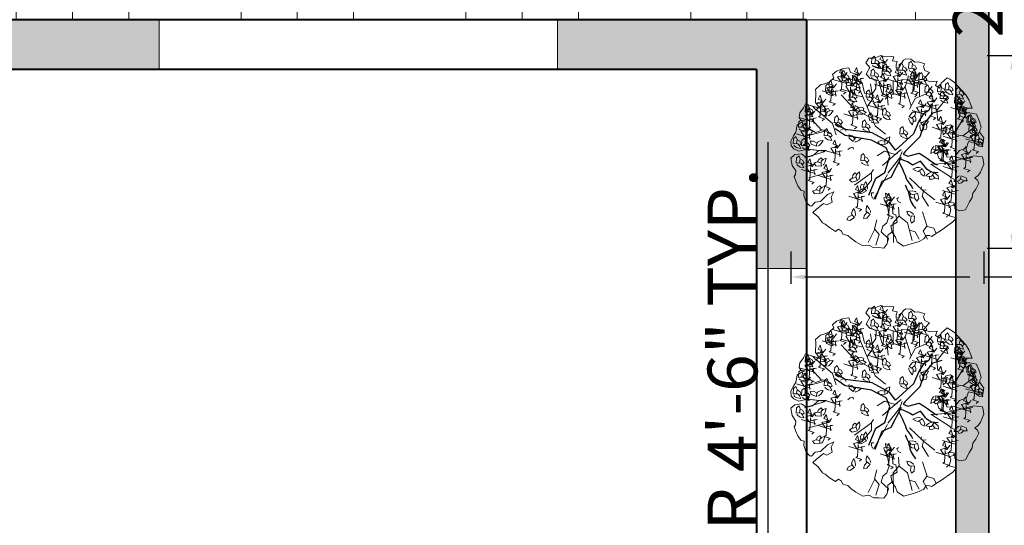
# Model space of a CAD drawing. Units: inches. Extents: x 2337 to 3570, y 1258 to 1938.
# Tile 27 of 30: x 3293 to 3471, y 1673 to 1764. Entities that reach past the tile are written whole.
import ezdxf

# ---------------------------------------------------------------- set-up
doc = ezdxf.new("R2010")
doc.units = ezdxf.units.IN
for name, color, linetype, lineweight in [('A-ANNO-DIMS', 2, 'Continuous', 18), ('A-FLOR-EDGE', 8, 'Continuous', 20), ('A-FLOR-PATT', 252, 'Continuous', 13), ('A-GLAZ', 4, 'Continuous', 18), ('A-WALL', 7, 'Continuous', 40), ('ARBOL', 74, 'Continuous', 13), ('C-PROP', 7, 'Continuous', 35)]:
    doc.layers.add(name, color=color, linetype=linetype, lineweight=lineweight)
doc.layers.add('A-WALL-PATT', color=18, linetype='Continuous', lineweight=13, true_color=0x000000)
doc.layers.add('C-PROP-PATT', color=251, linetype='Continuous', lineweight=13, true_color=0x636466)
doc.layers.add('TALLO', color=36, linetype='Continuous')
doc.styles.get("Standard").update_dxf_attribs({"font": 'arial.ttf'})
doc.dimstyles.new('ISO-25', dxfattribs={"dimtxt": 9, "dimasz": 2.5, "dimexe": 1.25, "dimexo": 0.625, "dimtad": 1, "dimdec": 1, "dimlunit": 3, "dimtxsty": 'Standard', "dimcen": 2.5, "dimadec": 0, "dimazin": 0, "dimtfac": 1, "dimtdec": 1, "dimtmove": 0, "dimatfit": 3, "dimfxl": 1, "dimarcsym": 0})

# ---------------------------------------------------------------- blocks, each defined once
blk = doc.blocks.new('fresno')
at = {"layer": 'ARBOL'}
for p, q in [((2.96, 0.991), (3.575, 1.984)), ((-3.638, 1.194), (-4.164, 1.76)), ((-1.151, -0.932), (-1.99, -1.556)), ((-0.974, -3.757), (-1.31, -4.423))]:
    blk.add_line(p, q, dxfattribs=at)
blk.add_lwpolyline([(0.823, 4.745), (0.566, 4.764), (0.459, 4.687), (0.336, 4.518), (0.233, 4.322), (0.087, 4.298), (0.091, 4.464), (0.14, 4.621), (-0.09, 4.659), (-0.033, 4.863), (-0.264, 4.901), (-0.483, 4.866), (-0.686, 4.924), (-1.021, 4.801), (-1.288, 4.8), (-1.431, 4.563), (-1.234, 4.327), (-1.406, 4), (-1.205, 3.778), (-0.909, 3.705), (-0.931, 3.283), (-1.122, 2.983), (-1.491, 3.043), (-1.619, 3.562), (-1.9, 3.727), (-1.851, 3.982), (-2.197, 4.084), (-2.278, 4.31), (-2.543, 4.283), (-2.896, 4.152), (-3.091, 3.971), (-3.022, 3.817), (-3.244, 3.617), (-3.424, 3.528), (-3.697, 3.455), (-3.946, 3.236), (-3.922, 3.09), (-3.94, 2.548), (-3.617, 2.495), (-3.927, 2.19), (-4.062, 2.379), (-4.443, 2.512), (-4.546, 2.316), (-4.73, 2.062), (-4.767, 1.832), (-4.671, 1.698), (-4.486, 1.667), (-4.693, 1.559), (-4.854, 1.444), (-4.934, 1.102), (-5.037, 0.905), (-5.175, 0.644), (-5.166, 0.406), (-5.024, 0.264), (-4.781, 0.153), (-4.363, 0.249), (-4.014, 0.215), (-3.783, 0.177), (-3.46, 0.124), (-3.733, 0.051), (-4.132, -0.073), (-4.404, -0.146), (-4.639, 0.011), (-4.977, -0.028), (-5.172, -0.209), (-5.113, -0.574), (-4.921, -0.843), (-4.951, -1.027), (-5.012, -1.112), (-4.95, -1.311), (-4.83, -1.592), (-4.676, -1.807), (-4.518, -1.856), (-4.529, -2.068), (-4.417, -2.394), (-4.236, -2.59), (-4.143, -2.605), (-3.967, -2.397), (-3.703, -2.37), (-3.339, -2.027), (-3.032, -1.889), (-3.169, -2.15), (-3.115, -2.396), (-3.376, -2.542), (-3.552, -2.466), (-3.909, -2.762), (-4.077, -2.924), (-3.804, -3.135), (-3.592, -3.43), (-3.461, -3.499), (-3.253, -3.676), (-2.953, -3.867), (-2.792, -3.752), (-2.642, -3.848), (-2.572, -4.001), (-2.323, -4.066), (-2.18, -4.208), (-1.926, -4.392), (-1.58, -4.591), (-1.288, -4.545), (-1.027, -4.683), (-0.788, -4.675), (-0.531, -4.693), (-0.382, -4.505), (-0.29, -4.236), (-0.66, -3.891), (-0.588, -3.595), (-0.374, -3.441), (-0.267, -3.079), (-0.368, -2.541), (-0.208, -2.426), (-0.099, -2.633), (-0.087, -2.991), (0.071, -3.04), (0.129, -3.405), (-0.185, -3.59), (-0.119, -3.909), (0.055, -4.151), (0.136, -4.377), (0.456, -4.596), (0.828, -4.491), (1.227, -4.368), (1.461, -4.241), (1.583, -4.071), (1.748, -4.075), (1.86, -4.117), (2.101, -3.944), (2.308, -3.836), (2.925, -3.393), (3.101, -3.185), (2.74, -3.078), (2.812, -2.782), (2.769, -2.61), (3.015, -2.555), (3.012, -2.721), (3.254, -2.832), (3.546, -2.785), (3.752, -2.393), (3.882, -2.177), (3.92, -1.947), (4.069, -1.758), (4.214, -1.451), (4.144, -1.297), (4.021, -1.182), (4.182, -1.067), (4.304, -0.897), (4.464, -0.497), (4.429, -0.279), (4.406, -0.133), (3.964, -0.083), (3.074, -0.315), (2.582, -0.424), (2.217, -0.197), (2.136, 0.029), (2.462, 0.141), (2.628, -0.147), (3.012, -0.116), (3.249, 0.177), (3.602, 0.308), (3.701, 0.623), (4.089, 0.535), (4.404, 0.436), (4.464, 0.805), (4.272, 1.074), (4.267, 1.193), (4.336, 1.324), (4.243, 1.623), (4.092, 2.003), (3.769, 2.057), (3.485, 2.056), (3.642, 2.291), (3.88, 2.299), (3.71, 2.706), (3.563, 2.967), (3.201, 3.358), (3.001, 3.581), (2.766, 3.738), (2.635, 3.807), (2.332, 3.549), (2.268, 3.299), (2.052, 3.429), (2.136, 3.652), (1.798, 3.613), (1.437, 3.72), (1.755, 4.071), (1.513, 4.182), (1.451, 4.381), (1.519, 4.512), (1.204, 4.611), (1.012, 4.596)], close=True, dxfattribs=at)
for points in [[(-0.346, 4.735), (-0.501, 4.528), (-0.605, 4.545), (-0.605, 4.614), (-0.519, 4.563), (-0.622, 4.925), (-0.726, 4.735), (-0.484, 4.632), (-0.622, 4.58), (-0.829, 4.528), (-0.657, 4.27), (-1.053, 4.39), (-0.363, 4.183), (-0.381, 4.114), (-0.415, 4.373), (-0.26, 4.39), (-0.57, 4.321), (-0.588, 4.476), (-0.622, 3.89), (-0.708, 3.839), (-0.398, 3.735), (-0.467, 3.701), (-0.519, 3.649)], [(-1.104, 4.45), (-1.063, 4.399), (-0.939, 4.325), (-0.757, 4.285), (-0.82, 4.431), (-0.903, 4.527), (-1.075, 4.533), (-1.143, 4.521), (-1.126, 4.792), (-1.002, 4.891), (-0.939, 4.738), (-0.975, 4.535)], [(-0.935, 4.717), (-0.809, 4.65), (-0.736, 4.529), (-0.824, 4.459)], [(-0.521, 4.069), (-0.48, 4.018), (-0.356, 3.944), (-0.174, 3.904), (-0.237, 4.051), (-0.32, 4.146), (-0.492, 4.152), (-0.56, 4.14), (-0.543, 4.411), (-0.419, 4.511), (-0.356, 4.357), (-0.392, 4.154)], [(0.263, 4.114), (0.304, 4.063), (0.429, 3.989), (0.611, 3.948), (0.547, 4.095), (0.465, 4.191), (0.293, 4.197), (0.225, 4.185), (0.242, 4.456), (0.366, 4.555), (0.428, 4.402), (0.393, 4.199)], [(0.734, 4.203), (0.775, 4.152), (0.9, 4.078), (1.082, 4.038), (1.018, 4.185), (0.936, 4.281), (0.763, 4.287), (0.696, 4.274), (0.712, 4.546), (0.837, 4.645), (0.899, 4.491), (0.863, 4.289)], [(0.904, 4.471), (1.029, 4.404), (1.102, 4.282), (1.015, 4.212)], [(-2.368, 4.073), (-2.523, 3.866), (-2.627, 3.883), (-2.627, 3.952), (-2.541, 3.9), (-2.644, 4.262), (-2.748, 4.073), (-2.506, 3.969), (-2.644, 3.918), (-2.851, 3.866), (-2.679, 3.607), (-3.075, 3.728), (-2.385, 3.521), (-2.403, 3.452), (-2.437, 3.711), (-2.282, 3.728), (-2.592, 3.659), (-2.61, 3.814), (-2.644, 3.228), (-2.73, 3.176), (-2.42, 3.073), (-2.489, 3.038), (-2.541, 2.987)], [(-2.629, 3.733), (-2.588, 3.682), (-2.463, 3.608), (-2.281, 3.568), (-2.345, 3.715), (-2.427, 3.81), (-2.6, 3.816), (-2.667, 3.804), (-2.651, 4.075), (-2.526, 4.175), (-2.464, 4.021), (-2.5, 3.818)], [(-2.459, 4), (-2.334, 3.933), (-2.261, 3.812), (-2.348, 3.742)], [(-1.623, 4.132), (-1.778, 3.925), (-1.882, 3.942), (-1.882, 4.011), (-1.795, 3.959), (-1.899, 4.321), (-2.002, 4.132), (-1.761, 4.028), (-1.899, 3.977), (-2.106, 3.925), (-1.933, 3.666), (-2.33, 3.787), (-1.64, 3.58), (-1.657, 3.511), (-1.692, 3.77), (-1.537, 3.787), (-1.847, 3.718), (-1.864, 3.873), (-1.899, 3.287), (-1.985, 3.235), (-1.675, 3.132), (-1.744, 3.097), (-1.795, 3.046)], [(-1.149, 3.822), (-1.108, 3.771), (-0.983, 3.697), (-0.802, 3.657), (-0.865, 3.804), (-0.948, 3.9), (-1.12, 3.906), (-1.188, 3.893), (-1.171, 4.165), (-1.047, 4.264), (-0.984, 4.111), (-1.02, 3.908)], [(-0.287, 3.833), (-0.442, 3.626), (-0.546, 3.643), (-0.546, 3.712), (-0.46, 3.661), (-0.563, 4.023), (-0.667, 3.833), (-0.425, 3.73), (-0.563, 3.678), (-0.77, 3.626), (-0.598, 3.367), (-0.995, 3.488), (-0.304, 3.281), (-0.322, 3.212), (-0.356, 3.471), (-0.201, 3.488), (-0.511, 3.419), (-0.529, 3.574), (-0.563, 2.988), (-0.649, 2.936), (-0.339, 2.833), (-0.408, 2.799), (-0.46, 2.747)], [(-0.98, 4.09), (-0.854, 4.023), (-0.781, 3.901), (-0.869, 3.831)], [(-0.352, 4.337), (-0.226, 4.269), (-0.153, 4.148), (-0.241, 4.078)], [(0.413, 4.08), (0.258, 3.873), (0.154, 3.89), (0.154, 3.959), (0.241, 3.908), (0.137, 4.27), (0.034, 4.08), (0.275, 3.977), (0.137, 3.925), (-0.07, 3.873), (0.103, 3.614), (-0.294, 3.735), (0.396, 3.528), (0.379, 3.459), (0.344, 3.718), (0.499, 3.735), (0.189, 3.666), (0.172, 3.821), (0.137, 3.235), (0.051, 3.183), (0.361, 3.08), (0.292, 3.046), (0.241, 2.994)], [(0.433, 4.381), (0.558, 4.314), (0.631, 4.193), (0.544, 4.122)], [(1.189, 3.942), (1.034, 3.735), (0.931, 3.752), (0.931, 3.821), (1.017, 3.77), (0.913, 4.132), (0.81, 3.942), (1.051, 3.839), (0.913, 3.787), (0.706, 3.735), (0.879, 3.477), (0.482, 3.597), (1.172, 3.39), (1.155, 3.321), (1.12, 3.58), (1.276, 3.597), (0.965, 3.528), (0.948, 3.683), (0.913, 3.097), (0.827, 3.046), (1.138, 2.942), (1.069, 2.908), (1.017, 2.856)], [(1.259, 4.08), (1.103, 3.873), (1, 3.89), (1, 3.959), (1.086, 3.908), (0.982, 4.27), (0.879, 4.08), (1.12, 3.977), (0.982, 3.925), (0.775, 3.873), (0.948, 3.614), (0.551, 3.735), (1.241, 3.528), (1.224, 3.459), (1.189, 3.718), (1.345, 3.735), (1.034, 3.666), (1.017, 3.821), (0.982, 3.235), (0.896, 3.183), (1.207, 3.08), (1.138, 3.046), (1.086, 2.994)], [(1.25, 3.643), (1.291, 3.592), (1.416, 3.518), (1.597, 3.478), (1.534, 3.625), (1.451, 3.721), (1.279, 3.727), (1.211, 3.714), (1.228, 3.985), (1.352, 4.085), (1.415, 3.931), (1.379, 3.729)], [(-2.898, 3.511), (-3.053, 3.304), (-3.157, 3.321), (-3.157, 3.39), (-3.071, 3.339), (-3.174, 3.701), (-3.278, 3.511), (-3.036, 3.408), (-3.174, 3.356), (-3.381, 3.304), (-3.209, 3.046), (-3.605, 3.166), (-2.915, 2.959), (-2.932, 2.89), (-2.967, 3.149), (-2.812, 3.166), (-3.122, 3.097), (-3.14, 3.253), (-3.174, 2.666), (-3.26, 2.615), (-2.95, 2.511), (-3.019, 2.477), (-3.071, 2.425)], [(-3.413, 3.083), (-3.373, 3.032), (-3.248, 2.958), (-3.066, 2.918), (-3.129, 3.065), (-3.212, 3.161), (-3.384, 3.167), (-3.452, 3.154), (-3.435, 3.425), (-3.311, 3.525), (-3.248, 3.371), (-3.284, 3.169)], [(-1.951, 3.597), (-2.106, 3.39), (-2.209, 3.408), (-2.209, 3.477), (-2.123, 3.425), (-2.227, 3.787), (-2.33, 3.597), (-2.089, 3.494), (-2.227, 3.442), (-2.434, 3.39), (-2.261, 3.132), (-2.658, 3.252), (-1.968, 3.046), (-1.985, 2.977), (-2.02, 3.235), (-1.864, 3.252), (-2.175, 3.183), (-2.192, 3.339), (-2.227, 2.752), (-2.313, 2.701), (-2.002, 2.597), (-2.071, 2.563), (-2.123, 2.511)], [(-2.068, 3.464), (-2.027, 3.413), (-1.903, 3.339), (-1.721, 3.299), (-1.784, 3.446), (-1.867, 3.542), (-2.039, 3.547), (-2.107, 3.535), (-2.09, 3.806), (-1.966, 3.906), (-1.903, 3.752), (-1.939, 3.55)], [(-1.899, 3.732), (-1.773, 3.664), (-1.7, 3.543), (-1.788, 3.473)], [(-1.367, 2.367), (-1.081, 2.78), (-1.193, 3.514)], [(-0.923, 3.449), (-0.951, 3.425), (-0.93, 3.313)], [(-0.358, 2.895), (-0.615, 3.037), (-0.783, 3.596)], [(-0.063, 3.671), (-0.069, 3.151), (-0.364, 2.965), (-0.319, 2.449)], [(0.558, 3.402), (0.403, 3.195), (0.299, 3.212), (0.299, 3.281), (0.386, 3.23), (0.282, 3.592), (0.179, 3.402), (0.42, 3.299), (0.282, 3.247), (0.075, 3.195), (0.248, 2.936), (-0.149, 3.057), (0.541, 2.85), (0.524, 2.781), (0.489, 3.04), (0.644, 3.057), (0.334, 2.988), (0.317, 3.143), (0.282, 2.557), (0.196, 2.505), (0.506, 2.402), (0.437, 2.368), (0.386, 2.316)], [(0.837, 2.414), (0.533, 3.352), (0.697, 3.906)], [(1.259, 2.882), (1.254, 3.446), (1.381, 3.636)], [(1.419, 3.911), (1.545, 3.844), (1.618, 3.722), (1.53, 3.652)], [(1.564, 3.016), (1.605, 2.965), (1.729, 2.891), (1.911, 2.851), (1.848, 2.998), (1.765, 3.094), (1.593, 3.099), (1.525, 3.087), (1.542, 3.358), (1.666, 3.458), (1.729, 3.304), (1.693, 3.102)], [(2.191, 3.038), (2.232, 2.987), (2.357, 2.913), (2.539, 2.873), (2.475, 3.02), (2.393, 3.116), (2.221, 3.122), (2.153, 3.109), (2.17, 3.381), (2.294, 3.48), (2.356, 3.326), (2.321, 3.124)], [(2.573, 3.128), (2.613, 3.077), (2.738, 3.003), (2.92, 2.963), (2.857, 3.11), (2.774, 3.205), (2.602, 3.211), (2.534, 3.199), (2.551, 3.47), (2.675, 3.57), (2.738, 3.416), (2.702, 3.214)], [(-3.244, 3.351), (-3.118, 3.284), (-3.045, 3.162), (-3.133, 3.092)], [(-1.112, 1.773), (-2.014, 2.265), (-2.654, 2.957)], [(-2.225, 2.77), (-2.184, 2.718), (-2.06, 2.645), (-1.878, 2.604), (-1.941, 2.751), (-2.024, 2.847), (-2.196, 2.853), (-2.264, 2.84), (-2.247, 3.112), (-2.123, 3.211), (-2.06, 3.058), (-2.096, 2.855)], [(-1.575, 2.854), (-2.052, 2.969), (-2.2, 3.178)], [(-2.056, 3.037), (-1.93, 2.97), (-1.857, 2.849), (-1.945, 2.778)], [(-0.448, 1), (-0.961, 1.419), (-1.784, 3.341)], [(-1.373, 2.77), (-1.332, 2.718), (-1.208, 2.645), (-1.026, 2.604), (-1.089, 2.751), (-1.172, 2.847), (-1.344, 2.853), (-1.412, 2.84), (-1.395, 3.112), (-1.271, 3.211), (-1.208, 3.058), (-1.244, 2.855)], [(-0.57, 2.77), (-0.726, 2.563), (-0.829, 2.58), (-0.829, 2.649), (-0.743, 2.597), (-0.846, 2.959), (-0.95, 2.77), (-0.708, 2.666), (-0.846, 2.615), (-1.053, 2.563), (-0.881, 2.304), (-1.278, 2.425), (-0.588, 2.218), (-0.605, 2.149), (-0.639, 2.408), (-0.484, 2.425), (-0.795, 2.356), (-0.812, 2.511), (-0.846, 1.925), (-0.933, 1.873), (-0.622, 1.77), (-0.691, 1.735), (-0.743, 1.684)], [(-1.204, 3.037), (-1.078, 2.97), (-1.005, 2.849), (-1.093, 2.778)], [(-0.41, 3.035), (-0.387, 2.974), (-0.291, 2.865), (-0.131, 2.771), (-0.146, 2.93), (-0.195, 3.047), (-0.357, 3.106), (-0.425, 3.115), (-0.325, 3.368), (-0.176, 3.424), (-0.164, 3.258), (-0.261, 3.077)], [(-0.166, 3.238), (-0.068, 3.135), (-0.036, 2.997), (-0.141, 2.957)], [(0.746, 2.242), (1.034, 2.786), (1.584, 3.019), (1.879, 3.374)], [(2.121, 2.804), (1.966, 2.597), (1.862, 2.615), (1.862, 2.683), (1.949, 2.632), (1.845, 2.994), (1.742, 2.804), (1.983, 2.701), (1.845, 2.649), (1.638, 2.597), (1.811, 2.339), (1.414, 2.459), (2.104, 2.252), (2.087, 2.184), (2.052, 2.442), (2.207, 2.459), (1.897, 2.39), (1.88, 2.546), (1.845, 1.959), (1.759, 1.908), (2.069, 1.804), (2, 1.77), (1.949, 1.718)], [(1.733, 3.284), (1.859, 3.216), (1.932, 3.095), (1.844, 3.025)], [(2.326, 2.702), (2.367, 2.651), (2.492, 2.577), (2.673, 2.537), (2.61, 2.684), (2.527, 2.78), (2.355, 2.786), (2.287, 2.773), (2.304, 3.045), (2.428, 3.144), (2.491, 2.99), (2.455, 2.788)], [(2.361, 3.306), (2.486, 3.239), (2.559, 3.117), (2.472, 3.047)], [(2.495, 2.97), (2.621, 2.903), (2.694, 2.781), (2.606, 2.711)], [(2.742, 3.396), (2.868, 3.328), (2.941, 3.207), (2.853, 3.137)], [(3.111, 2.904), (3.152, 2.853), (3.276, 2.779), (3.458, 2.739), (3.395, 2.886), (3.312, 2.981), (3.14, 2.987), (3.072, 2.975), (3.089, 3.246), (3.213, 3.346), (3.276, 3.192), (3.24, 2.99)], [(3.28, 3.172), (3.406, 3.104), (3.479, 2.983), (3.391, 2.913)], [(-4.422, 2.03), (-4.381, 1.979), (-4.257, 1.905), (-4.075, 1.865), (-4.138, 2.012), (-4.221, 2.108), (-4.393, 2.114), (-4.461, 2.101), (-4.444, 2.372), (-4.32, 2.472), (-4.257, 2.318), (-4.293, 2.116)], [(-3.434, 2.752), (-3.59, 2.546), (-3.693, 2.563), (-3.693, 2.632), (-3.607, 2.58), (-3.71, 2.942), (-3.814, 2.752), (-3.572, 2.649), (-3.71, 2.597), (-3.917, 2.546), (-3.745, 2.287), (-4.142, 2.408), (-3.452, 2.201), (-3.469, 2.132), (-3.503, 2.39), (-3.348, 2.408), (-3.659, 2.339), (-3.676, 2.494), (-3.71, 1.908), (-3.797, 1.856), (-3.486, 1.753), (-3.555, 1.718), (-3.607, 1.666)], [(-3.468, 1.85), (-3.409, 2.222), (-3.628, 2.505)], [(-1.817, 2.351), (-1.972, 2.144), (-2.075, 2.162), (-2.075, 2.231), (-1.989, 2.179), (-2.093, 2.541), (-2.196, 2.351), (-1.955, 2.248), (-2.093, 2.196), (-2.3, 2.144), (-2.127, 1.886), (-2.524, 2.006), (-1.834, 1.8), (-1.851, 1.731), (-1.886, 1.989), (-1.73, 2.006), (-2.041, 1.937), (-2.058, 2.093), (-2.093, 1.506), (-2.179, 1.455), (-1.868, 1.351), (-1.937, 1.317), (-1.989, 1.265)], [(1.586, 2.528), (1.431, 2.321), (1.327, 2.339), (1.327, 2.408), (1.414, 2.356), (1.31, 2.718), (1.207, 2.528), (1.448, 2.425), (1.31, 2.373), (1.103, 2.321), (1.276, 2.063), (0.879, 2.184), (1.569, 1.977), (1.552, 1.908), (1.517, 2.166), (1.673, 2.184), (1.362, 2.115), (1.345, 2.27), (1.31, 1.684), (1.224, 1.632), (1.535, 1.528), (1.466, 1.494), (1.414, 1.442)], [(2.171, 1.674), (2.121, 2.172), (2.689, 2.898)], [(3.519, 2.666), (3.363, 2.459), (3.26, 2.477), (3.26, 2.546), (3.346, 2.494), (3.243, 2.856), (3.139, 2.666), (3.381, 2.563), (3.243, 2.511), (3.036, 2.459), (3.208, 2.201), (2.811, 2.321), (3.501, 2.115), (3.484, 2.046), (3.45, 2.304), (3.605, 2.321), (3.294, 2.252), (3.277, 2.408), (3.243, 1.821), (3.156, 1.77), (3.467, 1.666), (3.398, 1.632), (3.346, 1.58)], [(3.043, 2.478), (3.084, 2.427), (3.209, 2.353), (3.391, 2.313), (3.327, 2.46), (3.245, 2.556), (3.073, 2.562), (3.005, 2.549), (3.022, 2.82), (3.146, 2.92), (3.208, 2.766), (3.173, 2.564)], [(3.178, 2.165), (3.219, 2.113), (3.344, 2.04), (3.525, 1.999), (3.462, 2.146), (3.379, 2.242), (3.207, 2.248), (3.139, 2.236), (3.156, 2.507), (3.28, 2.606), (3.343, 2.453), (3.307, 2.25)], [(3.213, 2.746), (3.338, 2.679), (3.411, 2.557), (3.324, 2.487)], [(-3.986, 2.149), (-4.142, 1.942), (-4.245, 1.959), (-4.245, 2.028), (-4.159, 1.977), (-4.262, 2.339), (-4.366, 2.149), (-4.124, 2.046), (-4.262, 1.994), (-4.47, 1.942), (-4.297, 1.684), (-4.694, 1.804), (-4.004, 1.597), (-4.021, 1.528), (-4.055, 1.787), (-3.9, 1.804), (-4.211, 1.735), (-4.228, 1.89), (-4.262, 1.304), (-4.349, 1.253), (-4.038, 1.149), (-4.107, 1.115), (-4.159, 1.063)], [(-4.253, 2.298), (-4.127, 2.231), (-4.054, 2.109), (-4.142, 2.039)], [(-2.916, 0.958), (-3.096, 1.528), (-3.871, 2.197)], [(-3.331, 1.905), (-3.269, 1.928), (-3.161, 2.024), (-3.066, 2.184), (-3.226, 2.169), (-3.342, 2.121), (-3.401, 1.958), (-3.41, 1.89), (-3.663, 1.99), (-3.719, 2.139), (-3.554, 2.151), (-3.372, 2.054)], [(-3.533, 2.149), (-3.43, 2.247), (-3.292, 2.279), (-3.252, 2.174)], [(-1.786, 2.007), (-1.722, 1.99), (-1.578, 2.003), (-1.407, 2.078), (-1.545, 2.159), (-1.668, 2.188), (-1.811, 2.092), (-1.859, 2.042), (-2.004, 2.271), (-1.962, 2.425), (-1.821, 2.337), (-1.731, 2.152)], [(-1.806, 2.323), (-1.665, 2.343), (-1.534, 2.287), (-1.564, 2.179)], [(-1.164, 1.612), (-1.109, 1.576), (-0.967, 1.544), (-0.782, 1.562), (-0.888, 1.682), (-0.996, 1.748), (-1.162, 1.7), (-1.222, 1.667), (-1.29, 1.93), (-1.203, 2.063), (-1.096, 1.937), (-1.067, 1.733)], [(-0.566, 1.873), (-0.525, 1.822), (-0.4, 1.748), (-0.219, 1.708), (-0.282, 1.855), (-0.365, 1.951), (-0.537, 1.957), (-0.605, 1.944), (-0.588, 2.216), (-0.464, 2.315), (-0.401, 2.162), (-0.437, 1.959)], [(-0.397, 2.141), (-0.271, 2.074), (-0.198, 1.952), (-0.286, 1.882)], [(0.72, 1.798), (0.723, 1.733), (0.781, 1.6), (0.904, 1.46), (0.939, 1.616), (0.929, 1.742), (0.793, 1.848), (0.73, 1.878), (0.904, 2.088), (1.062, 2.095), (1.023, 1.934), (0.875, 1.791)], [(3.245, 1.963), (3.286, 1.912), (3.411, 1.838), (3.593, 1.798), (3.529, 1.945), (3.447, 2.041), (3.274, 2.046), (3.206, 2.034), (3.223, 2.305), (3.347, 2.405), (3.41, 2.251), (3.374, 2.049)], [(3.347, 2.432), (3.473, 2.365), (3.546, 2.244), (3.458, 2.173)], [(3.415, 2.231), (3.54, 2.163), (3.613, 2.042), (3.525, 1.972)], [(3.716, 1.537), (3.757, 1.486), (3.882, 1.412), (4.063, 1.372), (4, 1.519), (3.917, 1.615), (3.745, 1.621), (3.677, 1.608), (3.694, 1.88), (3.818, 1.979), (3.881, 1.825), (3.845, 1.623)], [(-4.193, 1.356), (-4.349, 1.149), (-4.452, 1.166), (-4.452, 1.235), (-4.366, 1.184), (-4.469, 1.546), (-4.573, 1.356), (-4.331, 1.253), (-4.469, 1.201), (-4.677, 1.149), (-4.504, 0.89), (-4.901, 1.011), (-4.211, 0.804), (-4.228, 0.735), (-4.262, 0.994), (-4.107, 1.011), (-4.418, 0.942), (-4.435, 1.097), (-4.469, 0.511), (-4.556, 0.459), (-4.245, 0.356), (-4.314, 0.322), (-4.366, 0.27)], [(-4.759, 1.269), (-4.718, 1.217), (-4.593, 1.144), (-4.411, 1.103), (-4.475, 1.25), (-4.557, 1.346), (-4.729, 1.352), (-4.797, 1.339), (-4.78, 1.611), (-4.656, 1.71), (-4.594, 1.557), (-4.629, 1.354)], [(-4.589, 1.536), (-4.464, 1.469), (-4.391, 1.348), (-4.478, 1.277)], [(-2.965, 1.493), (-2.924, 1.441), (-2.799, 1.368), (-2.618, 1.327), (-2.681, 1.474), (-2.764, 1.57), (-2.936, 1.576), (-3.004, 1.564), (-2.987, 1.835), (-2.863, 1.934), (-2.8, 1.781), (-2.836, 1.578)], [(-2.796, 1.76), (-2.67, 1.693), (-2.597, 1.572), (-2.685, 1.501)], [(-1.575, 1.269), (-1.534, 1.217), (-1.409, 1.144), (-1.228, 1.103), (-1.291, 1.25), (-1.373, 1.346), (-1.546, 1.352), (-1.614, 1.339), (-1.597, 1.611), (-1.473, 1.71), (-1.41, 1.557), (-1.446, 1.354)], [(-1.406, 1.536), (-1.28, 1.469), (-1.207, 1.348), (-1.295, 1.277)], [(-1.085, 1.919), (-0.945, 1.893), (-0.838, 1.801), (-0.9, 1.707)], [(1.014, 1.915), (1.077, 1.787), (1.064, 1.646), (0.952, 1.64)], [(1.283, 1.469), (1.266, 1.405), (1.279, 1.261), (1.354, 1.09), (1.435, 1.228), (1.464, 1.351), (1.368, 1.494), (1.318, 1.542), (1.547, 1.687), (1.7, 1.645), (1.613, 1.504), (1.428, 1.414)], [(1.599, 1.489), (1.618, 1.348), (1.563, 1.217), (1.455, 1.247)], [(2.587, 1.684), (2.432, 1.477), (2.328, 1.494), (2.328, 1.563), (2.414, 1.511), (2.311, 1.873), (2.207, 1.684), (2.449, 1.58), (2.311, 1.528), (2.104, 1.477), (2.276, 1.218), (1.88, 1.339), (2.57, 1.132), (2.552, 1.063), (2.518, 1.321), (2.673, 1.339), (2.363, 1.27), (2.345, 1.425), (2.311, 0.839), (2.225, 0.787), (2.535, 0.684), (2.466, 0.649), (2.414, 0.597)], [(3.649, 1.515), (3.69, 1.464), (3.814, 1.39), (3.996, 1.35), (3.933, 1.497), (3.85, 1.592), (3.678, 1.598), (3.61, 1.586), (3.627, 1.857), (3.751, 1.957), (3.814, 1.803), (3.778, 1.601)], [(3.761, 1.112), (3.802, 1.061), (3.926, 0.987), (4.108, 0.947), (4.045, 1.093), (3.962, 1.189), (3.79, 1.195), (3.722, 1.183), (3.739, 1.454), (3.863, 1.553), (3.926, 1.4), (3.89, 1.197)], [(3.818, 1.783), (3.944, 1.715), (4.017, 1.594), (3.929, 1.524)], [(3.885, 1.805), (4.011, 1.738), (4.084, 1.616), (3.996, 1.546)], [(-3.354, 1.176), (-4.529, 0.864)], [(-3.192, 1.017), (-3.578, 1.215), (-3.949, 1.081), (-4.398, 1.339)], [(-3.481, 0.843), (-3.44, 0.792), (-3.315, 0.718), (-3.133, 0.678), (-3.197, 0.825), (-3.279, 0.92), (-3.451, 0.926), (-3.519, 0.914), (-3.502, 1.185), (-3.378, 1.285), (-3.316, 1.131), (-3.351, 0.928)], [(-3.311, 1.111), (-3.186, 1.043), (-3.113, 0.922), (-3.2, 0.852)], [(-2.703, 1.201), (-2.575, 1.263), (-2.433, 1.251), (-2.428, 1.139)], [(0.308, 0.933), (0.349, 0.881), (0.474, 0.807), (0.656, 0.767), (0.592, 0.914), (0.51, 1.01), (0.337, 1.016), (0.27, 1.003), (0.286, 1.275), (0.411, 1.374), (0.473, 1.221), (0.437, 1.018)], [(0.478, 1.2), (0.603, 1.133), (0.676, 1.011), (0.589, 0.941)], [(2.479, 1.34), (2.443, 1.285), (2.411, 1.143), (2.429, 0.958), (2.549, 1.064), (2.615, 1.172), (2.567, 1.338), (2.534, 1.398), (2.797, 1.466), (2.93, 1.379), (2.804, 1.272), (2.6, 1.243)], [(3.139, 1.235), (2.984, 1.028), (2.88, 1.046), (2.88, 1.115), (2.967, 1.063), (2.863, 1.425), (2.759, 1.235), (3.001, 1.132), (2.863, 1.08), (2.656, 1.028), (2.828, 0.77), (2.432, 0.891), (3.122, 0.684), (3.105, 0.615), (3.07, 0.873), (3.225, 0.891), (2.915, 0.822), (2.897, 0.977), (2.863, 0.391), (2.777, 0.339), (3.087, 0.235), (3.018, 0.201), (2.967, 0.149)], [(2.786, 1.261), (2.76, 1.121), (2.668, 1.014), (2.574, 1.076)], [(2.808, 1.015), (3.422, 0.918), (3.422, 0.918), (3.748, 0.794), (4.154, 1.111)], [(4.01, 1.36), (3.422, 0.918)], [(4.26, 1.115), (4.105, 0.908), (4.002, 0.925), (4.002, 0.994), (4.088, 0.942), (3.984, 1.304), (3.881, 1.115), (4.122, 1.011), (3.984, 0.959), (3.777, 0.908), (3.95, 0.649), (3.553, 0.77), (4.243, 0.563), (4.226, 0.494), (4.191, 0.753), (4.347, 0.77), (4.036, 0.701), (4.019, 0.856), (3.984, 0.27), (3.898, 0.218), (4.209, 0.115), (4.14, 0.08), (4.088, 0.029)], [(3.93, 1.379), (4.056, 1.312), (4.129, 1.191), (4.041, 1.121)], [(-5.028, 0.44), (-4.987, 0.388), (-4.862, 0.315), (-4.68, 0.274), (-4.744, 0.421), (-4.826, 0.517), (-4.998, 0.523), (-5.066, 0.511), (-5.049, 0.782), (-4.925, 0.881), (-4.863, 0.728), (-4.898, 0.525)], [(-4.858, 0.707), (-4.733, 0.64), (-4.66, 0.519), (-4.747, 0.448)], [(-4.602, 0.35), (-4.561, 0.299), (-4.436, 0.225), (-4.254, 0.185), (-4.318, 0.332), (-4.4, 0.428), (-4.572, 0.433), (-4.64, 0.421), (-4.623, 0.692), (-4.499, 0.792), (-4.437, 0.638), (-4.472, 0.436)], [(-4.432, 0.618), (-4.307, 0.55), (-4.234, 0.429), (-4.321, 0.359)], [(-3.824, 0.404), (-3.763, 0.427), (-3.654, 0.523), (-3.559, 0.683), (-3.719, 0.668), (-3.835, 0.62), (-3.894, 0.457), (-3.903, 0.389), (-4.156, 0.489), (-4.212, 0.638), (-4.047, 0.65), (-3.865, 0.553)], [(-2.698, 0.509), (-2.854, 0.302), (-2.957, 0.319), (-2.957, 0.388), (-2.871, 0.336), (-2.974, 0.698), (-3.078, 0.509), (-2.836, 0.405), (-2.974, 0.353), (-3.182, 0.302), (-3.009, 0.043), (-3.406, 0.164), (-2.716, -0.043), (-2.733, -0.112), (-2.767, 0.147), (-2.612, 0.164), (-2.923, 0.095), (-2.94, 0.25), (-2.974, -0.336), (-3.061, -0.388), (-2.75, -0.491), (-2.819, -0.526), (-2.871, -0.577)], [(-1.981, 0.615), (-1.915, 0.618), (-1.782, 0.676), (-1.643, 0.799), (-1.799, 0.834), (-1.925, 0.824), (-2.031, 0.688), (-2.061, 0.626), (-2.27, 0.799), (-2.278, 0.958), (-2.117, 0.918), (-1.974, 0.77)], [(-0.397, 0.517), (-0.346, 0.557), (-0.272, 0.682), (-0.232, 0.864), (-0.379, 0.801), (-0.474, 0.718), (-0.48, 0.546), (-0.468, 0.478), (-0.739, 0.495), (-0.838, 0.619), (-0.685, 0.682), (-0.482, 0.646)], [(2.639, 0.58), (2.483, 0.373), (2.38, 0.391), (2.38, 0.46), (2.466, 0.408), (2.363, 0.77), (2.259, 0.58), (2.501, 0.477), (2.363, 0.425), (2.156, 0.373), (2.328, 0.115), (1.931, 0.235), (2.621, 0.029), (2.604, -0.04), (2.57, 0.218), (2.725, 0.235), (2.414, 0.166), (2.397, 0.322), (2.363, -0.265), (2.276, -0.316), (2.587, -0.42), (2.518, -0.454), (2.466, -0.506)], [(2.708, 0.563), (2.552, 0.356), (2.449, 0.373), (2.449, 0.442), (2.535, 0.391), (2.432, 0.753), (2.328, 0.563), (2.57, 0.46), (2.432, 0.408), (2.225, 0.356), (2.397, 0.097), (2, 0.218), (2.69, 0.011), (2.673, -0.058), (2.639, 0.201), (2.794, 0.218), (2.483, 0.149), (2.466, 0.304), (2.432, -0.282), (2.345, -0.334), (2.656, -0.437), (2.587, -0.471), (2.535, -0.523)], [(4.075, 0.529), (4.116, 0.478), (4.24, 0.404), (4.422, 0.364), (4.359, 0.511), (4.276, 0.607), (4.104, 0.613), (4.036, 0.6), (4.053, 0.871), (4.177, 0.971), (4.24, 0.817), (4.204, 0.615)], [(4.244, 0.797), (4.37, 0.73), (4.443, 0.608), (4.355, 0.538)], [(-3.394, 0.18), (-3.77, 0.182), (-4.532, 0.27)], [(-3.77, 0.182), (-4.09, -0.088), (-4.494, -0.18)], [(-2.322, 0.222), (-2.219, 0.321), (-2.081, 0.353), (-2.042, 0.248)], [(-1.642, -0.412), (-1.601, -0.463), (-1.477, -0.537), (-1.295, -0.577), (-1.358, -0.43), (-1.441, -0.334), (-1.613, -0.328), (-1.681, -0.341), (-1.664, -0.069), (-1.54, 0.03), (-1.477, -0.124), (-1.513, -0.326)], [(0.03, -0.026), (-0.491, 0.154), (-0.871, -0.08)], [(-0.596, -0.564), (0.03, -0.026), (0.339, 0.235)], [(0.38, 0.131), (0.248, -0.21), (-0.33, -0.951)], [(1.978, 0.384), (1.927, 0.343), (1.853, 0.218), (1.813, 0.036), (1.96, 0.1), (2.056, 0.182), (2.061, 0.355), (2.049, 0.422), (2.32, 0.406), (2.42, 0.281), (2.266, 0.219), (2.064, 0.254)], [(2.246, 0.214), (2.178, 0.089), (2.057, 0.016), (1.987, 0.103)], [(3.829, 0.184), (3.674, -0.023), (3.57, -0.006), (3.57, 0.063), (3.657, 0.011), (3.553, 0.373), (3.45, 0.184), (3.691, 0.08), (3.553, 0.029), (3.346, -0.023), (3.519, -0.282), (3.122, -0.161), (3.812, -0.368), (3.795, -0.437), (3.76, -0.178), (3.915, -0.161), (3.605, -0.23), (3.588, -0.075), (3.553, -0.661), (3.467, -0.713), (3.777, -0.816), (3.708, -0.851), (3.657, -0.902)], [(-4.871, -0.524), (-4.83, -0.575), (-4.705, -0.649), (-4.523, -0.689), (-4.587, -0.542), (-4.669, -0.446), (-4.841, -0.44), (-4.909, -0.453), (-4.893, -0.181), (-4.768, -0.082), (-4.706, -0.236), (-4.741, -0.438)], [(-4.701, -0.256), (-4.576, -0.323), (-4.503, -0.445), (-4.59, -0.515)], [(-3.952, -0.42), (-4.107, -0.627), (-4.211, -0.609), (-4.211, -0.54), (-4.124, -0.592), (-4.228, -0.23), (-4.331, -0.42), (-4.09, -0.523), (-4.228, -0.575), (-4.435, -0.627), (-4.262, -0.885), (-4.659, -0.765), (-3.969, -0.971), (-3.986, -1.04), (-4.021, -0.782), (-3.866, -0.765), (-4.176, -0.834), (-4.193, -0.678), (-4.228, -1.265), (-4.314, -1.316), (-4.004, -1.42), (-4.073, -1.454), (-4.124, -1.506)], [(-3.58, -0.559), (-3.529, -0.518), (-3.455, -0.393), (-3.415, -0.211), (-3.562, -0.275), (-3.658, -0.357), (-3.664, -0.53), (-3.651, -0.597), (-3.923, -0.581), (-4.022, -0.456), (-3.868, -0.394), (-3.666, -0.43)], [(-3.848, -0.389), (-3.781, -0.264), (-3.659, -0.191), (-3.589, -0.278)], [(-1.473, -0.144), (-1.347, -0.211), (-1.274, -0.333), (-1.362, -0.403)], [(1.846, -0.51), (2.605, -0.469), (3.129, -0.637)], [(3.139, -0.282), (2.984, -0.489), (2.88, -0.471), (2.88, -0.402), (2.967, -0.454), (2.863, -0.092), (2.759, -0.282), (3.001, -0.385), (2.863, -0.437), (2.656, -0.489), (2.828, -0.747), (2.432, -0.627), (3.122, -0.834), (3.105, -0.902), (3.07, -0.644), (3.225, -0.627), (2.915, -0.696), (2.897, -0.54), (2.863, -1.127), (2.777, -1.178), (3.087, -1.282), (3.018, -1.316), (2.967, -1.368)], [(-3.195, -0.824), (-3.267, -0.898), (-4.285, -1.185)], [(-3.141, -0.713), (-3.296, -0.92), (-3.4, -0.902), (-3.4, -0.834), (-3.314, -0.885), (-3.417, -0.523), (-3.521, -0.713), (-3.279, -0.816), (-3.417, -0.868), (-3.624, -0.92), (-3.452, -1.178), (-3.848, -1.058), (-3.158, -1.265), (-3.175, -1.333), (-3.21, -1.075), (-3.055, -1.058), (-3.365, -1.127), (-3.383, -0.971), (-3.417, -1.558), (-3.503, -1.609), (-3.193, -1.713), (-3.262, -1.747), (-3.314, -1.799)], [(-1.794, -1.268), (-1.758, -1.214), (-1.726, -1.072), (-1.744, -0.887), (-1.865, -0.993), (-1.93, -1.101), (-1.883, -1.266), (-1.85, -1.327), (-2.113, -1.395), (-2.246, -1.307), (-2.119, -1.2), (-1.916, -1.172)], [(-2.101, -1.19), (-2.076, -1.05), (-1.983, -0.943), (-1.889, -1.004)], [(-1.047, -0.767), (-1.151, -0.913), (-1.144, -1.307), (-1.61, -1.871)], [(1.304, -0.681), (1.241, -0.664), (1.097, -0.678), (0.926, -0.752), (1.064, -0.833), (1.187, -0.862), (1.33, -0.766), (1.377, -0.716), (1.523, -0.945), (1.481, -1.099), (1.34, -1.011), (1.25, -0.826)], [(1.903, -0.903), (1.837, -0.905), (1.704, -0.963), (1.565, -1.086), (1.721, -1.122), (1.847, -1.111), (1.953, -0.975), (1.983, -0.913), (2.192, -1.086), (2.2, -1.245), (2.039, -1.205), (1.896, -1.057)], [(1.822, -0.495), (2.859, -1.165)], [(-1.361, -1.756), (-1.343, -1.693), (-1.357, -1.548), (-1.431, -1.377), (-1.513, -1.515), (-1.542, -1.638), (-1.445, -1.781), (-1.395, -1.829), (-1.625, -1.974), (-1.778, -1.932), (-1.691, -1.791), (-1.506, -1.701)], [(-0.346, -1.024), (-1.05, -2.251)], [(0.748, -1.185), (1.452, -1.855), (2.021, -2.292)], [(2.02, -1.197), (1.891, -1.259), (1.75, -1.247), (1.745, -1.134)], [(3.105, -1.471), (2.949, -1.678), (2.846, -1.661), (2.846, -1.592), (2.932, -1.644), (2.829, -1.282), (2.725, -1.471), (2.967, -1.575), (2.829, -1.627), (2.621, -1.678), (2.794, -1.937), (2.397, -1.816), (3.087, -2.023), (3.07, -2.092), (3.036, -1.833), (3.191, -1.816), (2.88, -1.885), (2.863, -1.73), (2.829, -2.316), (2.742, -2.368), (3.053, -2.471), (2.984, -2.506), (2.932, -2.558)], [(3.253, -1.094), (3.192, -1.117), (3.083, -1.213), (2.988, -1.374), (3.148, -1.359), (3.264, -1.31), (3.323, -1.148), (3.332, -1.079), (3.585, -1.179), (3.641, -1.328), (3.476, -1.34), (3.294, -1.244)], [(3.455, -1.338), (3.352, -1.437), (3.214, -1.469), (3.175, -1.364)], [(-3.648, -1.948), (-3.596, -1.907), (-3.523, -1.782), (-3.482, -1.6), (-3.629, -1.664), (-3.725, -1.746), (-3.731, -1.919), (-3.719, -1.986), (-3.99, -1.97), (-4.089, -1.845), (-3.936, -1.783), (-3.733, -1.819)], [(-3.915, -1.778), (-3.848, -1.653), (-3.727, -1.58), (-3.656, -1.667)], [(-1.571, -1.764), (-1.726, -1.971), (-1.83, -1.954), (-1.83, -1.885), (-1.744, -1.937), (-1.847, -1.575), (-1.951, -1.764), (-1.709, -1.868), (-1.847, -1.92), (-2.054, -1.971), (-1.882, -2.23), (-2.278, -2.109), (-1.588, -2.316), (-1.605, -2.385), (-1.64, -2.127), (-1.485, -2.109), (-1.795, -2.178), (-1.813, -2.023), (-1.847, -2.609), (-1.933, -2.661), (-1.623, -2.764), (-1.692, -2.799), (-1.744, -2.851)], [(-1.677, -1.776), (-1.696, -1.635), (-1.641, -1.504), (-1.533, -1.534)], [(-1.092, -2.202), (-1.154, -2.074), (-1.142, -1.933), (-1.03, -1.928)], [(-0.001, -2.144), (-0.156, -2.351), (-0.26, -2.333), (-0.26, -2.264), (-0.174, -2.316), (-0.277, -1.954), (-0.381, -2.144), (-0.139, -2.247), (-0.277, -2.299), (-0.484, -2.351), (-0.312, -2.609), (-0.708, -2.489), (-0.018, -2.695), (-0.035, -2.764), (-0.07, -2.506), (0.085, -2.489), (-0.225, -2.558), (-0.243, -2.402), (-0.277, -2.989), (-0.363, -3.04), (-0.053, -3.144), (-0.122, -3.178), (-0.174, -3.23)], [(-0.161, -2.225), (-0.184, -2.163), (-0.28, -2.055), (-0.44, -1.96), (-0.425, -2.12), (-0.376, -2.236), (-0.214, -2.295), (-0.146, -2.304), (-0.246, -2.557), (-0.395, -2.613), (-0.407, -2.448), (-0.31, -2.266)], [(1.086, -1.899), (1.031, -1.863), (0.89, -1.831), (0.704, -1.849), (0.81, -1.969), (0.918, -2.035), (1.084, -1.987), (1.145, -1.954), (1.212, -2.218), (1.125, -2.35), (1.018, -2.224), (0.989, -2.02)], [(1.593, -1.781), (1.452, -1.801), (1.322, -1.746), (1.352, -1.637)], [(1.452, -1.855), (1.379, -2.105), (1.698, -2.609)], [(2.777, -2.058), (2.621, -2.264), (2.518, -2.247), (2.518, -2.178), (2.604, -2.23), (2.501, -1.868), (2.397, -2.058), (2.639, -2.161), (2.501, -2.213), (2.294, -2.264), (2.466, -2.523), (2.069, -2.402), (2.759, -2.609), (2.742, -2.678), (2.708, -2.42), (2.863, -2.402), (2.552, -2.471), (2.535, -2.316), (2.501, -2.902), (2.414, -2.954), (2.725, -3.057), (2.656, -3.092), (2.604, -3.144)], [(-0.405, -2.427), (-0.503, -2.324), (-0.535, -2.186), (-0.43, -2.146)], [(0.319, -2.428), (0.193, -2.361), (0.12, -2.239), (0.208, -2.169)], [(1.007, -2.206), (0.867, -2.181), (0.76, -2.088), (0.822, -1.994)], [(-1.966, -3.1), (-1.949, -3.037), (-1.962, -2.892), (-2.037, -2.722), (-2.118, -2.859), (-2.147, -2.982), (-2.051, -3.125), (-2.001, -3.173), (-2.23, -3.319), (-2.383, -3.277), (-2.296, -3.136), (-2.111, -3.046)], [(-1.201, -2.914), (-1.204, -2.849), (-1.262, -2.716), (-1.385, -2.576), (-1.42, -2.732), (-1.41, -2.858), (-1.274, -2.964), (-1.212, -2.994), (-1.385, -3.204), (-1.544, -3.211), (-1.504, -3.05), (-1.356, -2.907)], [(0.201, -2.655), (0.24, -3.105), (0.657, -3.436), (0.886, -4.322)], [(0.959, -3.012), (0.918, -2.961), (0.793, -2.887), (0.612, -2.847), (0.675, -2.994), (0.758, -3.089), (0.93, -3.095), (0.998, -3.083), (0.981, -3.354), (0.857, -3.453), (0.794, -3.3), (0.83, -3.097)], [(1.399, -2.886), (1.63, -3.612), (1.964, -3.708), (2.084, -3.964)], [(-0.923, -4.549), (-0.768, -4.012), (-0.99, -3.737), (-0.872, -3.28)], [(0.238, -3.084), (-0.067, -3.438), (-0.048, -4.412)], [(-0.059, -3.851), (-0.336, -4.054), (-0.355, -4.41)], [(0.752, -3.801), (1.042, -3.878), (1.233, -4.25)], [(1.625, -3.596), (1.438, -3.858), (1.657, -4.248)]]:
    blk.add_lwpolyline(points, dxfattribs=at)
for p in [(-0.308, 0.101), (0.124, 0.027)]:
    blk.add_point(p, dxfattribs=at)
at = {"layer": 'TALLO'}
for points in [[(1.829, 2.5), (1.722, 2.184), (1.454, 2.012), (1.213, 1.639), (0.944, 1.008), (0.06, 0.204), (-0.234, 0.577), (-1.119, 1.065), (-2.458, 1.237), (-2.941, 1.524)], [(2.364, 2.184), (1.909, 2.041), (1.507, 1.552), (1.266, 0.864), (0.542, 0.125), (0.433, 0.001), (0.662, -0.096), (1.228, 0.045), (1.455, -0.09), (1.644, -0.216), (1.8, -0.33), (1.931, -0.425), (2.042, -0.496), (2.141, -0.539)], [(-1.272, -2.047), (-0.931, -1.203), (-0.475, -0.916), (-0.234, -0.112), (-0.422, 0.318), (-1.146, 0.691), (-2.458, 0.921), (-2.967, 1.266)], [(2.177, -0.932), (2.008, -0.924), (1.873, -0.898), (1.766, -0.859), (1.682, -0.807), (1.613, -0.745), (1.554, -0.676), (1.499, -0.6), (1.442, -0.521), (1.376, -0.44), (1.298, -0.357), (0.908, -0.555), (0.791, -0.474), (0.647, -0.394), (0.474, -0.317), (0.265, -0.244), (0.226, -0.233), (0.328, -0.17), (-0.181, -1.175), (-0.637, -1.375), (-0.985, -2.265)], [(0.219, -0.386), (0.3, -0.544), (0.399, -0.753), (0.473, -0.922), (0.529, -1.057), (0.571, -1.164), (0.607, -1.251), (0.641, -1.324), (0.68, -1.389), (0.729, -1.454), (0.784, -1.525), (0.844, -1.61), (0.903, -1.717)], [(0.538, -1.536), (0.555, -1.568), (0.626, -1.728), (0.678, -1.871), (0.716, -2), (0.747, -2.115), (0.773, -2.219), (0.802, -2.314), (0.837, -2.401), (0.883, -2.483), (0.936, -2.562), (0.994, -2.642), (1.052, -2.727)]]:
    blk.add_lwpolyline(points, dxfattribs=at)
blk = doc.blocks.new('*D48')
at = {"layer": 'A-ANNO-DIMS', "color": 0, "lineweight": -2, "transparency": 16777216}
for p, q in [((3431.99, 1722.22), (3431.99, 1716.36)), ((3466.85, 1722.22), (3466.85, 1716.36)), ((3434.49, 1717.61), (3464.35, 1717.61)), ((3466.85, 1717.61), (3569.71, 1717.61))]:
    blk.add_line(p, q, dxfattribs=at)
at = {"layer": 'A-ANNO-DIMS', "color": 0, "transparency": 16777216}
for points in [[(3434.49, 1718.03), (3434.49, 1717.2), (3431.99, 1717.61)], [(3464.35, 1718.03), (3464.35, 1717.2), (3466.85, 1717.61)]]:
    blk.add_solid(points, dxfattribs=at)
at = {"layer": 'Defpoints', "color": 0, "transparency": 16777216}
for p in [(3431.99, 1722.84), (3466.85, 1722.84), (3466.85, 1717.61)]:
    blk.add_point(p, dxfattribs=at)
at = {"layer": 'A-ANNO-DIMS', "color": 0, "transparency": 16777216, "insert": (3519.53, 1722.76), "char_height": 9, "attachment_point": 5}
blk.add_mtext('TREE 2\'-11" TYP.', dxfattribs=at)
blk = doc.blocks.new('*D49')
at = {"layer": 'A-ANNO-DIMS', "color": 0, "lineweight": -2, "transparency": 16777216}
for p, q in [((3472.08, 1757.63), (3472.08, 1823.39)), ((3467.48, 1757.63), (3473.33, 1757.63)), ((3472.08, 1725.34), (3472.08, 1755.13)), ((3467.48, 1722.84), (3473.33, 1722.84))]:
    blk.add_line(p, q, dxfattribs=at)
at = {"layer": 'A-ANNO-DIMS', "color": 0, "transparency": 16777216}
for points in [[(3471.67, 1755.13), (3472.5, 1755.13), (3472.08, 1757.63)], [(3471.67, 1725.34), (3472.5, 1725.34), (3472.08, 1722.84)]]:
    blk.add_solid(points, dxfattribs=at)
at = {"layer": 'Defpoints', "color": 0, "transparency": 16777216}
for p in [(3466.85, 1757.63), (3472.08, 1757.63), (3466.85, 1722.84)]:
    blk.add_point(p, dxfattribs=at)
at = {"layer": 'A-ANNO-DIMS', "color": 0, "transparency": 16777216, "insert": (3466.94, 1791.76), "char_height": 9, "attachment_point": 5, "rotation": 90}
blk.add_mtext('2\'-11" TYP.', dxfattribs=at)
blk = doc.blocks.new('*D68')
at = {"layer": 'A-ANNO-DIMS', "color": 0, "lineweight": -2, "transparency": 16777216}
for p, q in [((3427.89, 1596.12), (3427.89, 1741.99)), ((3420.41, 1596.12), (3429.14, 1596.12)), ((3427.89, 1544.62), (3427.89, 1593.62)), ((3420.41, 1542.12), (3429.14, 1542.12))]:
    blk.add_line(p, q, dxfattribs=at)
at = {"layer": 'A-ANNO-DIMS', "color": 0, "transparency": 16777216}
for points in [[(3427.47, 1593.62), (3428.3, 1593.62), (3427.89, 1596.12)], [(3427.47, 1544.62), (3428.3, 1544.62), (3427.89, 1542.12)]]:
    blk.add_solid(points, dxfattribs=at)
at = {"layer": 'Defpoints', "color": 0, "transparency": 16777216}
for p in [(3419.79, 1596.12), (3427.89, 1596.12), (3419.79, 1542.12)]:
    blk.add_point(p, dxfattribs=at)
at = {"layer": 'A-ANNO-DIMS', "color": 0, "transparency": 16777216, "insert": (3422.6, 1670.3), "char_height": 9, "attachment_point": 5, "rotation": 90}
blk.add_mtext('SWING DOOR 4\'-6" TYP.', dxfattribs=at)

msp = doc.modelspace()

# ---------------------------------------------------------------- hatches: boundary and pattern name
at = {"layer": 'A-FLOR-PATT'}
h = msp.add_hatch(dxfattribs=at)
h.set_pattern_fill('AR-HBONE', color=256, scale=0.1, angle=45)
h.set_pattern_definition([(90, (-558.681, 0), (-10.16, 10.16), [30.48, -10.16]), (180, (-558.681, 10.16), (-10.16, 10.16), [30.48, -10.16])])
h.paths.add_polyline_path([(3281.79, 1810.12), (3281.79, 1764.12), (3434.79, 1764.12), (3461.79, 1764.12), (3461.79, 1779.12), (3464.79, 1779.12), (3464.79, 1875.12), (3461.79, 1875.12), (3461.79, 1887.12), (3233.79, 1887.12), (3233.79, 1857.12), (3243.79, 1857.12), (3243.79, 1810.12)])
h.paths.add_polyline_path([(3250.98, 1816.17), (3263.22, 1816.17), (3263.22, 1823.8), (3250.98, 1823.8)], flags=24)
h.paths.add_polyline_path([(3317.33, 1858.95), (3370.67, 1858.95), (3370.67, 1885.07), (3317.33, 1885.07)], flags=24)
at = {"layer": 'A-WALL-PATT'}
h = msp.add_hatch(color=256, dxfattribs=at)
h.dxf.hatch_style = 1
h.paths.add_polyline_path([(3233.79, 1857.12), (3017.79, 1857.12), (3017.79, 1824.12), (3026.79, 1824.12), (3026.79, 1848.12), (3233.79, 1848.12)])
h.paths.add_polyline_path([(3128.79, 1764.12), (3026.79, 1764.12), (3026.79, 1788.12), (3017.79, 1788.12), (3017.79, 1743.12), (3026.79, 1743.12), (3026.79, 1755.12), (3128.79, 1755.12)])
h.paths.add_polyline_path([(3245.79, 1761.12), (3245.79, 1764.12), (3164.79, 1764.12), (3164.79, 1755.12), (3170.79, 1755.12), (3170.79, 1701.12), (3224.79, 1701.12), (3224.79, 1605.12), (3233.79, 1605.12), (3233.79, 1713.12), (3224.79, 1713.12), (3224.79, 1707.12), (3176.79, 1707.12), (3176.79, 1755.12), (3224.79, 1755.12), (3224.79, 1749.12), (3233.79, 1749.12), (3233.79, 1755.12), (3245.79, 1755.12)])
h.paths.add_polyline_path([(3026.79, 1707.12), (3017.79, 1707.12), (3017.79, 1617.12), (3026.79, 1617.12), (3026.79, 1635.12), (3068.79, 1635.12), (3068.79, 1641.12), (3026.79, 1641.12)])
h.paths.add_polyline_path([(3104.79, 1551.12), (3026.79, 1551.12), (3026.79, 1569.12), (3017.79, 1569.12), (3017.79, 1518.12), (3026.79, 1518.12), (3026.79, 1542.12), (3104.79, 1542.12)])
h.paths.add_polyline_path([(3026.79, 1482.12), (3017.79, 1482.12), (3017.79, 1410.12), (3026.79, 1410.12)])
h.paths.add_polyline_path([(3188.79, 1350.12), (3152.79, 1350.12), (3152.79, 1380.12), (3146.79, 1380.12), (3146.79, 1350.12), (3026.79, 1350.12), (3026.79, 1374.12), (3017.79, 1374.12), (3017.79, 1341.12), (3188.79, 1341.12)])
h.paths.add_polyline_path([(3224.79, 1416.12), (3248.79, 1416.12), (3248.79, 1422.12), (3152.79, 1422.12), (3152.79, 1542.12), (3242.79, 1542.12), (3242.79, 1551.12), (3233.79, 1551.12), (3233.79, 1557.12), (3224.79, 1557.12), (3224.79, 1551.12), (3140.79, 1551.12), (3140.79, 1542.12), (3146.79, 1542.12), (3146.79, 1410.12), (3152.79, 1410.12), (3152.79, 1416.12), (3218.79, 1416.12), (3218.79, 1350.12), (3212.79, 1350.12), (3212.79, 1341.12), (3293.79, 1341.12), (3293.79, 1362.12), (3284.79, 1362.12), (3284.79, 1350.12), (3224.79, 1350.12)])
h.paths.add_polyline_path([(3293.79, 1434.12), (3284.79, 1434.12), (3284.79, 1422.12), (3278.79, 1422.12), (3278.79, 1416.12), (3284.79, 1416.12), (3284.79, 1386.12), (3293.79, 1386.12)], flags=17)
h.paths.add_polyline_path([(3293.79, 1542.12), (3314.79, 1542.12), (3314.79, 1551.12), (3278.79, 1551.12), (3278.79, 1545.12), (3278.79, 1542.12), (3284.79, 1542.12), (3284.79, 1482.12), (3293.79, 1482.12)])
h.paths.add_polyline_path([(3371.79, 1551.12), (3350.79, 1551.12), (3350.79, 1542.12), (3371.79, 1542.12), (3371.79, 1548.12)])
h.paths.add_polyline_path([(3434.79, 1647.12), (3425.79, 1647.12), (3425.79, 1551.12), (3419.79, 1551.12), (3419.79, 1548.12), (3419.79, 1542.12), (3434.79, 1542.12)])
h.paths.add_polyline_path([(3434.79, 1764.12), (3389.79, 1764.12), (3389.79, 1755.12), (3425.79, 1755.12), (3425.79, 1719.12), (3434.79, 1719.12)])
h.paths.add_polyline_path([(3317.79, 1764.12), (3281.79, 1764.12), (3281.79, 1755.12), (3317.79, 1755.12)])
at = {"layer": 'C-PROP-PATT'}
h = msp.add_hatch(color=256, dxfattribs=at)
h.dxf.hatch_style = 1
h.paths.add_polyline_path([(3467.79, 1893.12), (2987.79, 1893.12), (2987.79, 1293.12), (3293.79, 1293.12), (3293.79, 1299.12), (2993.79, 1299.12), (2993.79, 1887.12), (3461.79, 1887.12), (3461.79, 1875.12), (3467.79, 1875.12)])
h.paths.add_polyline_path([(3407.79, 1299.12), (3389.79, 1299.12), (3389.79, 1293.12), (3407.79, 1293.12)], flags=17)
h.paths.add_polyline_path([(3461.79, 1299.12), (3455.79, 1299.12), (3455.79, 1293.12), (3467.79, 1293.12), (3467.79, 1779.12), (3461.79, 1779.12)], flags=17)

# ---------------------------------------------------------------- linework, layer by layer
at = {"layer": 'A-FLOR-EDGE'}
msp.add_line((3434.79, 1764.12), (3461.79, 1764.12), dxfattribs=at)
at = {"layer": 'A-GLAZ'}
for p, q in [((3317.79, 1764.12), (3317.79, 1755.12)), ((3389.79, 1764.12), (3389.79, 1755.12)), ((3434.79, 1719.12), (3425.79, 1719.12))]:
    msp.add_line(p, q, dxfattribs=at)
at = {"layer": 'A-WALL'}
for p, q in [((3434.79, 1764.12), (3281.79, 1764.12)), ((3434.79, 1764.12), (3434.79, 1542.12)), ((3425.79, 1755.12), (3281.79, 1755.12)), ((3425.79, 1755.12), (3425.79, 1551.12))]:
    msp.add_line(p, q, dxfattribs=at)
at = {"layer": 'C-PROP'}
for p, q in [((3461.79, 1779.12), (3461.79, 1299.12)), ((3467.79, 1779.12), (3467.79, 1293.12))]:
    msp.add_line(p, q, dxfattribs=at)

# ---------------------------------------------------------------- block references
at = {"layer": 'ARBOL', "xscale": 3.617267037020409, "yscale": 3.617267037020409, "zscale": 3.617267037020409}
for p in [(3450.7, 1739.82), (3450.7, 1694.62)]:
    msp.add_blockref('fresno', p, dxfattribs=at)

# ---------------------------------------------------------------- dimensions: what is measured, and where the dimension line sits
at = {"layer": 'A-ANNO-DIMS'}
for base, p1, p2, text, picture, middle in [((3472.08, 1757.63), (3466.85, 1722.84), (3466.85, 1757.63), '<> TYP.', '*D49', (3466.94, 1791.76)), ((3427.89, 1596.12), (3419.79, 1542.12), (3419.79, 1596.12), 'SWING DOOR <> TYP.', '*D68', (3422.6, 1670.3))]:
    dim = msp.add_linear_dim(base=base, p1=p1, p2=p2, angle=90, text=text, dimstyle='ISO-25', override={"dimdec": 1, "dimlfac": 1, "dimrnd": 0, "dimzin": 1, "dimdsep": 46, "dimlunit": 4, "dimfrac": 2}, dxfattribs=at)
    dim.commit()
    dim.dimension.update_dxf_attribs({"geometry": picture, "text_midpoint": middle})
dim = msp.add_linear_dim(base=(3466.85, 1717.61), p1=(3431.99, 1722.84), p2=(3466.85, 1722.84), text='TREE <> TYP.', dimstyle='ISO-25', override={"dimdec": 1, "dimlfac": 1, "dimrnd": 0, "dimzin": 1, "dimdsep": 46, "dimlunit": 4, "dimfrac": 2}, dxfattribs=at)
dim.commit()
dim.dimension.update_dxf_attribs({"geometry": '*D48', "text_midpoint": (3519.53, 1722.76)})

doc.saveas('drawing.dxf')
